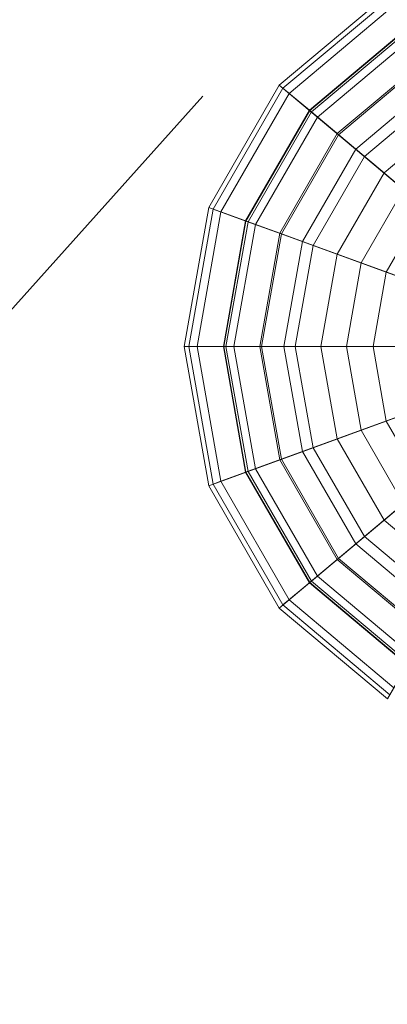
# Model space of a CAD drawing. Units: inches. Extents: x 375 to 1122, y 27 to 1069.
# Tile 138 of 155: x 731.16 to 732.384, y 896.928 to 900.205. Entities that reach past the tile are written whole.
import ezdxf

# ---------------------------------------------------------------- set-up
doc = ezdxf.new("R2010")
doc.units = ezdxf.units.IN
doc.layers.add('A-ANNO-DIMS', color=2, linetype='Continuous', lineweight=18)
doc.layers.add('Furniture', color=30, linetype='Continuous', lineweight=18)
doc.styles.get("Standard").update_dxf_attribs({"font": 'arial.ttf'})
doc.dimstyles.new('ISO-25', dxfattribs={"dimtxt": 12, "dimasz": 2.5, "dimexe": 1.5, "dimexo": 1.5, "dimtad": 1, "dimdec": 1, "dimlunit": 3, "dimtxsty": 'Standard', "dimblk": 'ARCHTICK', "dimcen": 2.5, "dimadec": 0, "dimazin": 0, "dimtfac": 1, "dimtdec": 1, "dimtmove": 0, "dimatfit": 3, "dimfxl": 1.5, "dimfxlon": 1, "dimarcsym": 0})

# ---------------------------------------------------------------- blocks, each defined once
blk = doc.blocks.new('A$C403C54AD')
blk.add_line((0.959313, 1.170619, -0.000599), (1.358468, 0.812559, -0.000599))
for points in [[(0.950832, 1.185986, -0.04658), (0.980157, 1.202917, -0.043501), (0.980157, 1.202917, -0.043501), (0.958391, 1.176977, -0.04658)], [(0.958391, 1.176977, -0.04658), (0.980157, 1.202917, -0.043501), (0.980157, 1.202917, -0.043501), (0.968576, 1.171097, -0.04658)], [(0.968576, 1.171097, -0.04658), (0.980157, 1.202917, -0.043501), (0.980157, 1.202917, -0.043501), (0.980157, 1.169055, -0.04658)], [(1.001923, 1.176977, -0.04658), (0.980157, 1.202917, -0.043501), (0.980157, 1.202917, -0.043501), (1.009483, 1.185986, -0.04658)], [(0.991739, 1.171097, -0.04658), (0.980157, 1.202917, -0.043501), (0.980157, 1.202917, -0.043501), (1.001923, 1.176977, -0.04658)], [(0.980157, 1.169055, -0.04658), (0.980157, 1.202917, -0.043501), (0.980157, 1.202917, -0.043501), (0.991739, 1.171097, -0.04658)], [(0.967847, 1.19581, -0.040074), (0.95366, 1.187619, -0.043349), (0.96049, 1.179479, -0.043349), (0.971021, 1.192029, -0.040074)], [(0.974434, 1.196096, 0.042248), (0.968505, 1.189031, 0.048884), (0.973957, 1.185883, 0.048884), (0.977112, 1.19455, 0.042248)], [(0.983203, 1.19455, 0.042248), (0.986357, 1.185883, 0.048884), (0.991809, 1.189031, 0.048884), (0.985881, 1.196096, 0.042248)], [(0.989294, 1.192029, -0.040074), (0.999824, 1.179479, -0.043349), (1.006655, 1.187619, -0.043349), (0.992467, 1.19581, -0.040074)], [(0.967072, 1.187323, 0.046697), (0.973653, 1.195166, 0.03933), (0.976696, 1.193409, 0.03933), (0.973195, 1.183788, 0.046697)], [(0.98712, 1.183788, 0.046697), (0.983618, 1.193409, 0.03933), (0.986661, 1.195166, 0.03933), (0.993243, 1.187323, 0.046697)], [(0.977112, 1.19455, 0.042248), (0.973957, 1.185883, 0.048884), (0.980157, 1.18479, 0.048884), (0.980157, 1.194013, 0.042248)], [(0.980157, 1.194013, 0.042248), (0.980157, 1.18479, 0.048884), (0.986357, 1.185883, 0.048884), (0.983203, 1.19455, 0.042248)], [(0.964459, 1.193854, 0.048884), (0.958842, 1.190611, 0.058276), (0.964336, 1.184063, 0.058276), (0.968505, 1.189031, 0.048884)], [(0.973195, 1.183788, 0.046697), (0.976696, 1.193409, 0.03933), (0.980157, 1.192799, 0.03933), (0.980157, 1.18256, 0.046697)], [(0.980157, 1.18256, 0.046697), (0.980157, 1.192799, 0.03933), (0.983618, 1.193409, 0.03933), (0.98712, 1.183788, 0.046697)], [(0.991809, 1.189031, 0.048884), (0.995978, 1.184063, 0.058276), (1.001473, 1.190611, 0.058276), (0.995856, 1.193854, 0.048884)], [(0.956408, 1.189206, 0.056929), (0.962527, 1.192739, 0.046697), (0.967072, 1.187323, 0.046697), (0.96253, 1.18191, 0.056929)], [(0.997785, 1.18191, 0.056929), (0.993243, 1.187323, 0.046697), (0.997787, 1.192739, 0.046697), (1.003907, 1.189206, 0.056929)], [(0.956282, 1.189133, 0.115599), (0.960688, 1.191677, 0.12581), (0.965707, 1.185696, 0.12581), (0.962436, 1.181798, 0.115599)], [(0.960688, 1.191677, 0.12581), (0.958022, 1.190138, 0.12581), (0.963728, 1.183338, 0.12581), (0.965707, 1.185696, 0.12581)], [(0.971021, 1.192029, -0.040074), (0.96049, 1.179479, -0.043349), (0.969693, 1.174166, -0.043349), (0.975296, 1.18956, -0.040074)], [(0.985019, 1.18956, -0.040074), (0.990622, 1.174166, -0.043349), (0.999824, 1.179479, -0.043349), (0.989294, 1.192029, -0.040074)], [(0.994608, 1.185696, 0.12581), (0.996587, 1.183338, 0.12581), (1.002293, 1.190138, 0.12581), (0.999627, 1.191677, 0.12581)], [(0.997878, 1.181798, 0.115599), (0.994608, 1.185696, 0.12581), (0.999627, 1.191677, 0.12581), (1.004033, 1.189133, 0.115599)], [(0.958022, 1.190138, 0.12581), (0.953695, 1.187639, 0.116404), (0.960516, 1.17951, 0.116404), (0.963728, 1.183338, 0.12581)], [(0.958842, 1.190611, 0.058276), (0.954418, 1.188057, 0.075423), (0.961053, 1.18015, 0.075423), (0.964336, 1.184063, 0.058276)], [(0.995978, 1.184063, 0.058276), (0.999261, 1.18015, 0.075423), (1.005896, 1.188057, 0.075423), (1.001473, 1.190611, 0.058276)], [(0.996587, 1.183338, 0.12581), (0.999798, 1.17951, 0.116404), (1.00662, 1.187639, 0.116404), (1.002293, 1.190138, 0.12581)], [(0.951762, 1.186523, 0.074938), (0.956408, 1.189206, 0.056929), (0.96253, 1.18191, 0.056929), (0.959081, 1.1778, 0.074938)], [(0.975296, 1.18956, -0.040074), (0.969693, 1.174166, -0.043349), (0.980157, 1.172321, -0.043349), (0.980157, 1.188703, -0.040074)], [(0.980157, 1.188703, -0.040074), (0.980157, 1.172321, -0.043349), (0.990622, 1.174166, -0.043349), (0.985019, 1.18956, -0.040074)], [(1.001233, 1.1778, 0.074938), (0.997785, 1.18191, 0.056929), (1.003907, 1.189206, 0.056929), (1.008553, 1.186523, 0.074938)], [(0.953848, 1.187728, 0.102963), (0.956282, 1.189133, 0.115599), (0.962436, 1.181798, 0.115599), (0.96063, 1.179646, 0.102963)], [(0.968505, 1.189031, 0.048884), (0.964336, 1.184063, 0.058276), (0.971739, 1.179789, 0.058276), (0.973957, 1.185883, 0.048884)], [(0.986357, 1.185883, 0.048884), (0.988575, 1.179789, 0.058276), (0.995978, 1.184063, 0.058276), (0.991809, 1.189031, 0.048884)], [(0.999684, 1.179646, 0.102963), (0.997878, 1.181798, 0.115599), (1.004033, 1.189133, 0.115599), (1.006466, 1.187728, 0.102963)], [(0.95366, 1.187619, -0.043349), (0.950832, 1.185986, -0.04658), (0.958391, 1.176977, -0.04658), (0.96049, 1.179479, -0.043349)], [(0.953695, 1.187639, 0.116404), (0.951177, 1.186186, 0.10318), (0.958647, 1.177283, 0.10318), (0.960516, 1.17951, 0.116404)], [(0.954418, 1.188057, 0.075423), (0.953848, 1.187728, 0.102963), (0.96063, 1.179646, 0.102963), (0.961053, 1.18015, 0.075423)], [(0.999261, 1.18015, 0.075423), (0.999684, 1.179646, 0.102963), (1.006466, 1.187728, 0.102963), (1.005896, 1.188057, 0.075423)], [(0.999798, 1.17951, 0.116404), (1.001667, 1.177283, 0.10318), (1.009137, 1.186186, 0.10318), (1.00662, 1.187639, 0.116404)], [(0.999824, 1.179479, -0.043349), (1.001923, 1.176977, -0.04658), (1.009483, 1.185986, -0.04658), (1.006655, 1.187619, -0.043349)], [(0.96253, 1.18191, 0.056929), (0.967072, 1.187323, 0.046697), (0.973195, 1.183788, 0.046697), (0.970778, 1.177147, 0.056929)], [(0.989537, 1.177147, 0.056929), (0.98712, 1.183788, 0.046697), (0.993243, 1.187323, 0.046697), (0.997785, 1.18191, 0.056929)], [(0.951177, 1.186186, 0.10318), (0.951762, 1.186523, 0.074938), (0.959081, 1.1778, 0.074938), (0.958647, 1.177283, 0.10318)], [(1.001667, 1.177283, 0.10318), (1.001233, 1.1778, 0.074938), (1.008553, 1.186523, 0.074938), (1.009137, 1.186186, 0.10318)], [(0.962436, 1.181798, 0.115599), (0.965707, 1.185696, 0.12581), (0.972468, 1.181792, 0.12581), (0.970728, 1.177011, 0.115599)], [(0.965707, 1.185696, 0.12581), (0.963728, 1.183338, 0.12581), (0.971415, 1.178899, 0.12581), (0.972468, 1.181792, 0.12581)], [(0.973957, 1.185883, 0.048884), (0.971739, 1.179789, 0.058276), (0.980157, 1.178304, 0.058276), (0.980157, 1.18479, 0.048884)], [(0.980157, 1.18479, 0.048884), (0.980157, 1.178304, 0.058276), (0.988575, 1.179789, 0.058276), (0.986357, 1.185883, 0.048884)], [(0.987846, 1.181792, 0.12581), (0.988899, 1.178899, 0.12581), (0.996587, 1.183338, 0.12581), (0.994608, 1.185696, 0.12581)], [(0.989586, 1.177011, 0.115599), (0.987846, 1.181792, 0.12581), (0.994608, 1.185696, 0.12581), (0.997878, 1.181798, 0.115599)], [(0.964336, 1.184063, 0.058276), (0.961053, 1.18015, 0.075423), (0.969992, 1.174989, 0.075423), (0.971739, 1.179789, 0.058276)], [(0.970778, 1.177147, 0.056929), (0.973195, 1.183788, 0.046697), (0.980157, 1.18256, 0.046697), (0.980157, 1.175494, 0.056929)], [(0.980157, 1.175494, 0.056929), (0.980157, 1.18256, 0.046697), (0.98712, 1.183788, 0.046697), (0.989537, 1.177147, 0.056929)], [(0.988575, 1.179789, 0.058276), (0.990322, 1.174989, 0.075423), (0.999261, 1.18015, 0.075423), (0.995978, 1.184063, 0.058276)], [(0.963728, 1.183338, 0.12581), (0.960516, 1.17951, 0.116404), (0.969706, 1.174204, 0.116404), (0.971415, 1.178899, 0.12581)], [(0.988899, 1.178899, 0.12581), (0.990608, 1.174204, 0.116404), (0.999798, 1.17951, 0.116404), (0.996587, 1.183338, 0.12581)], [(0.959081, 1.1778, 0.074938), (0.96253, 1.18191, 0.056929), (0.970778, 1.177147, 0.056929), (0.968943, 1.172106, 0.074938)], [(0.96063, 1.179646, 0.102963), (0.962436, 1.181798, 0.115599), (0.970728, 1.177011, 0.115599), (0.969767, 1.174371, 0.102963)], [(0.991372, 1.172106, 0.074938), (0.989537, 1.177147, 0.056929), (0.997785, 1.18191, 0.056929), (1.001233, 1.1778, 0.074938)], [(0.990547, 1.174371, 0.102963), (0.989586, 1.177011, 0.115599), (0.997878, 1.181798, 0.115599), (0.999684, 1.179646, 0.102963)], [(0.970728, 1.177011, 0.115599), (0.972468, 1.181792, 0.12581), (0.980157, 1.180436, 0.12581), (0.980157, 1.175348, 0.115599)], [(0.972468, 1.181792, 0.12581), (0.971415, 1.178899, 0.12581), (0.980157, 1.177358, 0.12581), (0.980157, 1.180436, 0.12581)], [(0.980157, 1.180436, 0.12581), (0.980157, 1.177358, 0.12581), (0.988899, 1.178899, 0.12581), (0.987846, 1.181792, 0.12581)], [(0.980157, 1.175348, 0.115599), (0.980157, 1.180436, 0.12581), (0.987846, 1.181792, 0.12581), (0.989586, 1.177011, 0.115599)], [(0.96049, 1.179479, -0.043349), (0.958391, 1.176977, -0.04658), (0.968576, 1.171097, -0.04658), (0.969693, 1.174166, -0.043349)], [(0.960516, 1.17951, 0.116404), (0.958647, 1.177283, 0.10318), (0.968712, 1.171472, 0.10318), (0.969706, 1.174204, 0.116404)], [(0.961053, 1.18015, 0.075423), (0.96063, 1.179646, 0.102963), (0.969767, 1.174371, 0.102963), (0.969992, 1.174989, 0.075423)], [(0.971739, 1.179789, 0.058276), (0.969992, 1.174989, 0.075423), (0.980157, 1.173197, 0.075423), (0.980157, 1.178304, 0.058276)], [(0.980157, 1.178304, 0.058276), (0.980157, 1.173197, 0.075423), (0.990322, 1.174989, 0.075423), (0.988575, 1.179789, 0.058276)], [(0.990322, 1.174989, 0.075423), (0.990547, 1.174371, 0.102963), (0.999684, 1.179646, 0.102963), (0.999261, 1.18015, 0.075423)], [(0.990608, 1.174204, 0.116404), (0.991602, 1.171472, 0.10318), (1.001667, 1.177283, 0.10318), (0.999798, 1.17951, 0.116404)], [(0.990622, 1.174166, -0.043349), (0.991739, 1.171097, -0.04658), (1.001923, 1.176977, -0.04658), (0.999824, 1.179479, -0.043349)], [(0.971415, 1.178899, 0.12581), (0.969706, 1.174204, 0.116404), (0.980157, 1.172361, 0.116404), (0.980157, 1.177358, 0.12581)], [(0.980157, 1.177358, 0.12581), (0.980157, 1.172361, 0.116404), (0.990608, 1.174204, 0.116404), (0.988899, 1.178899, 0.12581)], [(0.958647, 1.177283, 0.10318), (0.959081, 1.1778, 0.074938), (0.968943, 1.172106, 0.074938), (0.968712, 1.171472, 0.10318)], [(0.991602, 1.171472, 0.10318), (0.991372, 1.172106, 0.074938), (1.001233, 1.1778, 0.074938), (1.001667, 1.177283, 0.10318)], [(0.968943, 1.172106, 0.074938), (0.970778, 1.177147, 0.056929), (0.980157, 1.175494, 0.056929), (0.980157, 1.170129, 0.074938)], [(0.969767, 1.174371, 0.102963), (0.970728, 1.177011, 0.115599), (0.980157, 1.175348, 0.115599), (0.980157, 1.172539, 0.102963)], [(0.980157, 1.170129, 0.074938), (0.980157, 1.175494, 0.056929), (0.989537, 1.177147, 0.056929), (0.991372, 1.172106, 0.074938)], [(0.980157, 1.172539, 0.102963), (0.980157, 1.175348, 0.115599), (0.989586, 1.177011, 0.115599), (0.990547, 1.174371, 0.102963)], [(0.969992, 1.174989, 0.075423), (0.969767, 1.174371, 0.102963), (0.980157, 1.172539, 0.102963), (0.980157, 1.173197, 0.075423)], [(0.980157, 1.173197, 0.075423), (0.980157, 1.172539, 0.102963), (0.990547, 1.174371, 0.102963), (0.990322, 1.174989, 0.075423)], [(0.969693, 1.174166, -0.043349), (0.968576, 1.171097, -0.04658), (0.980157, 1.169055, -0.04658), (0.980157, 1.172321, -0.043349)], [(0.969706, 1.174204, 0.116404), (0.968712, 1.171472, 0.10318), (0.980157, 1.169454, 0.10318), (0.980157, 1.172361, 0.116404)], [(0.980157, 1.172361, 0.116404), (0.980157, 1.169454, 0.10318), (0.991602, 1.171472, 0.10318), (0.990608, 1.174204, 0.116404)], [(0.980157, 1.172321, -0.043349), (0.980157, 1.169055, -0.04658), (0.991739, 1.171097, -0.04658), (0.990622, 1.174166, -0.043349)], [(0.968712, 1.171472, 0.10318), (0.968943, 1.172106, 0.074938), (0.980157, 1.170129, 0.074938), (0.980157, 1.169454, 0.10318)], [(0.980157, 1.169454, 0.10318), (0.980157, 1.170129, 0.074938), (0.991372, 1.172106, 0.074938), (0.991602, 1.171472, 0.10318)]]:
    blk.add_3dface(points)
blk = doc.blocks.new('_ArchTick')
at = {"color": 0, "linetype": 'ByBlock', "const_width": 0.15}
blk.add_lwpolyline([(-0.5, -0.5), (0.5, 0.5)], dxfattribs=at)
blk = doc.blocks.new('*D73')
at = {"layer": 'A-ANNO-DIMS', "color": 0, "lineweight": -2, "transparency": 16777216}
for p, q in [((686.7573, 932.4277), (686.7573, 929.4277)), ((770.7573, 932.4277), (770.7573, 929.4277)), ((686.7573, 930.9277), (770.7573, 930.9277)), ((770.7573, 930.9277), (987.6096, 930.9277))]:
    blk.add_line(p, q, dxfattribs=at)
at = {"layer": 'Defpoints', "color": 0, "transparency": 16777216}
for p in [(686.7573, 943.5277), (770.7573, 943.5277), (770.7573, 930.9277)]:
    blk.add_point(p, dxfattribs=at)
at = {"layer": 'A-ANNO-DIMS', "color": 0, "lineweight": -2, "transparency": 16777216, "xscale": 2.5, "yscale": 2.5, "zscale": 2.5, "rotation": 180}
blk.add_blockref('_ArchTick', (686.7573, 930.9277), dxfattribs=at)
at = {"layer": 'A-ANNO-DIMS', "color": 0, "lineweight": -2, "transparency": 16777216, "xscale": 2.5, "yscale": 2.5, "zscale": 2.5}
blk.add_blockref('_ArchTick', (770.7573, 930.9277), dxfattribs=at)
at = {"layer": 'A-ANNO-DIMS', "color": 0, "transparency": 16777216, "insert": (880.4335, 937.7573), "char_height": 12, "attachment_point": 5}
blk.add_mtext('2-PANEL SLIDER 7\'-0" TYP.', dxfattribs=at)
blk = doc.blocks.new('*D88')
at = {"layer": 'A-ANNO-DIMS', "color": 0, "lineweight": -2, "transparency": 16777216}
for p, q in [((731.0073, 1052.5277), (731.0073, 1055.5277)), ((854.0073, 1052.5277), (854.0073, 1055.5277)), ((731.0073, 1054.0277), (854.0073, 1054.0277))]:
    blk.add_line(p, q, dxfattribs=at)
at = {"layer": 'Defpoints', "color": 0, "transparency": 16777216}
for p in [(854.0073, 1054.0277), (731.0073, 502.5277), (854.0073, 502.5277)]:
    blk.add_point(p, dxfattribs=at)
at = {"layer": 'A-ANNO-DIMS', "color": 0, "lineweight": -2, "transparency": 16777216, "xscale": 2.5, "yscale": 2.5, "zscale": 2.5, "rotation": 180}
blk.add_blockref('_ArchTick', (731.0073, 1054.0277), dxfattribs=at)
at = {"layer": 'A-ANNO-DIMS', "color": 0, "lineweight": -2, "transparency": 16777216, "xscale": 2.5, "yscale": 2.5, "zscale": 2.5}
blk.add_blockref('_ArchTick', (854.0073, 1054.0277), dxfattribs=at)
at = {"layer": 'A-ANNO-DIMS', "color": 0, "transparency": 16777216, "insert": (792.5073, 1060.7837), "char_height": 12, "attachment_point": 5}
blk.add_mtext('10\'-3"', dxfattribs=at)
blk = doc.blocks.new('*D91')
at = {"layer": 'A-ANNO-DIMS', "color": 0, "lineweight": -2, "transparency": 16777216}
for p, q in [((728.0073, 1052.5277), (728.0073, 1055.5277)), ((788.0073, 1052.5277), (788.0073, 1055.5277)), ((728.0073, 1054.0277), (788.0073, 1054.0277))]:
    blk.add_line(p, q, dxfattribs=at)
at = {"layer": 'Defpoints', "color": 0, "transparency": 16777216}
for p in [(788.0073, 1054.0277), (728.0073, 774.0277), (788.0073, 774.0277)]:
    blk.add_point(p, dxfattribs=at)
at = {"layer": 'A-ANNO-DIMS', "color": 0, "lineweight": -2, "transparency": 16777216, "xscale": 2.5, "yscale": 2.5, "zscale": 2.5, "rotation": 180}
blk.add_blockref('_ArchTick', (728.0073, 1054.0277), dxfattribs=at)
at = {"layer": 'A-ANNO-DIMS', "color": 0, "lineweight": -2, "transparency": 16777216, "xscale": 2.5, "yscale": 2.5, "zscale": 2.5}
blk.add_blockref('_ArchTick', (788.0073, 1054.0277), dxfattribs=at)
at = {"layer": 'A-ANNO-DIMS', "color": 0, "transparency": 16777216, "insert": (758.0073, 1060.7796), "char_height": 12, "attachment_point": 5}
blk.add_mtext('5\'-0"', dxfattribs=at)

msp = doc.modelspace()

# ---------------------------------------------------------------- block references
at = {"layer": 'Furniture', "xscale": 39.9918517141215, "yscale": 39.9918517141215, "zscale": 39.9918517141215, "rotation": 270}
msp.add_blockref('A$C403C54AD', (684.9549, 938.3156, 0.024), dxfattribs=at)

# ---------------------------------------------------------------- dimensions: what is measured, and where the dimension line sits
at = {"layer": 'A-ANNO-DIMS'}
for base, p1, p2, picture, middle in [((788.0073, 1054.0277), (728.0073, 774.0277), (788.0073, 774.0277), '*D91', (758.0073, 1060.7796)), ((854.0073, 1054.0277), (731.0073, 502.5277), (854.0073, 502.5277), '*D88', (792.5073, 1060.7837))]:
    dim = msp.add_linear_dim(base=base, p1=p1, p2=p2, dimstyle='ISO-25', override={"dimdec": 1, "dimlfac": 1, "dimrnd": 0, "dimzin": 1, "dimdsep": 46, "dimlunit": 4, "dimfrac": 2}, dxfattribs=at)
    dim.commit()
    dim.dimension.update_dxf_attribs({"geometry": picture, "text_midpoint": middle})
dim = msp.add_linear_dim(base=(770.7573, 930.9277), p1=(686.7573, 943.5277), p2=(770.7573, 943.5277), text='2-PANEL SLIDER <> TYP.', dimstyle='ISO-25', override={"dimdec": 1, "dimlfac": 1, "dimrnd": 0, "dimzin": 1, "dimdsep": 46, "dimlunit": 4, "dimfrac": 2}, dxfattribs=at)
dim.commit()
dim.dimension.update_dxf_attribs({"geometry": '*D73', "text_midpoint": (880.4335, 937.7573)})

doc.saveas('drawing.dxf')
